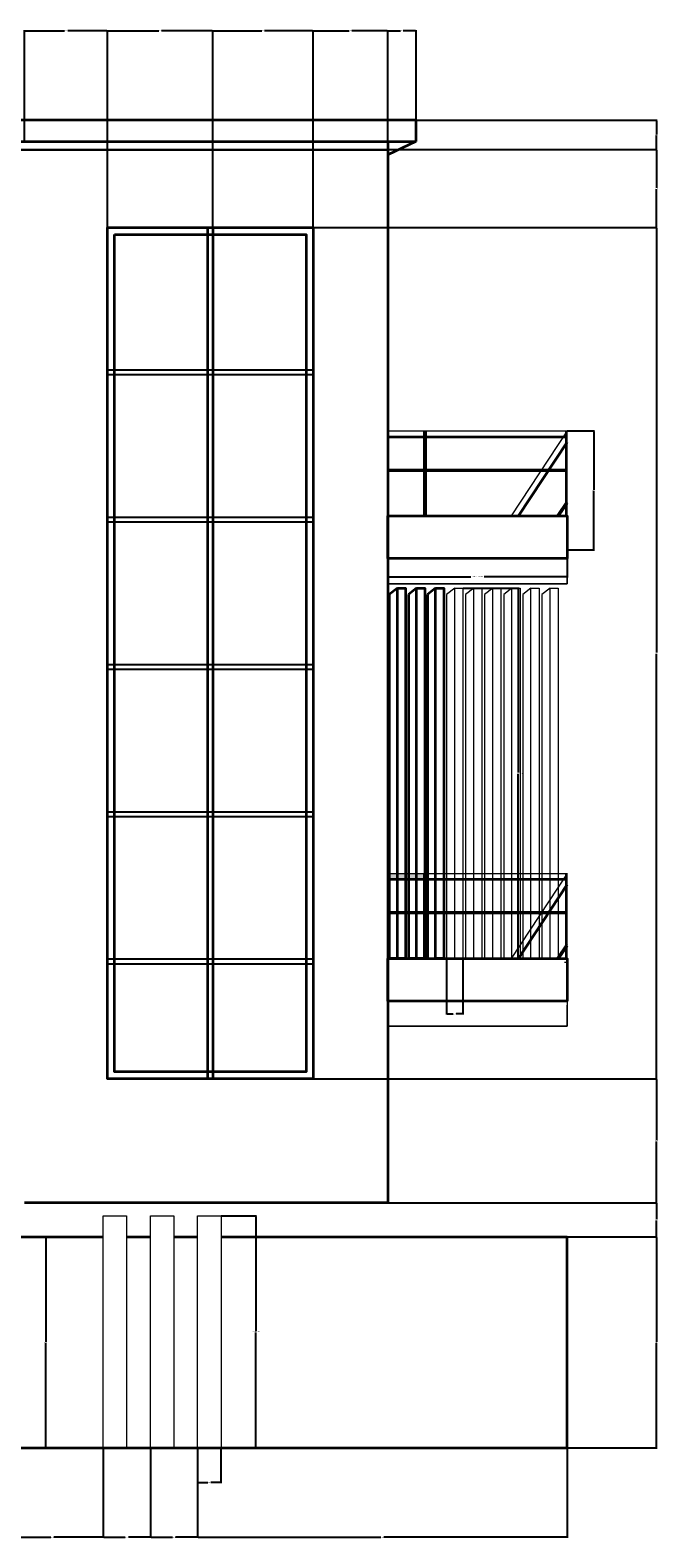
# Model space of a CAD drawing. Units: feet. Extents: x 2415 to 6174, y 866 to 1295.
# Tile 8 of 9: x 4309 to 4488, y 866 to 1295. Entities that reach past the tile are written whole.
import ezdxf

# ---------------------------------------------------------------- set-up
doc = ezdxf.new("R2010")
doc.units = ezdxf.units.FT
for name, color, linetype, lineweight in [('A-ANNO-DIMS', 2, 'Continuous', 18), ('A-ELEV', 7, 'Continuous', 35), ('A-ELEV-LOUV', 9, 'Continuous', 18), ('A-ELEV-PATT', 8, 'Continuous', 13), ('A-ELEV-RAIL', 3, 'Continuous', 18), ('A-GLAZ', 4, 'Continuous', 25)]:
    doc.layers.add(name, color=color, linetype=linetype, lineweight=lineweight)
doc.styles.get("Standard").update_dxf_attribs({"font": 'arial.ttf'})
doc.dimstyles.get("Standard").update_dxf_attribs({"dimtxt": 0.18, "dimasz": 0.18, "dimexe": 0.18, "dimexo": 0.0625, "dimgap": 0.09, "dimtad": 0, "dimtih": 1, "dimtoh": 1, "dimdec": 1, "dimzin": 0, "dimdsep": 46, "dimlunit": 3, "dimtxsty": 'Standard', "dimcen": 0.09, "dimadec": 0, "dimazin": 0, "dimtfac": 1, "dimtdec": 1, "dimtofl": 0, "dimtmove": 0, "dimatfit": 3, "dimfxl": 1, "dimtolj": 1, "dimtzin": 0, "dimarcsym": 0})

# ---------------------------------------------------------------- blocks, each defined once
blk = doc.blocks.new('LOUVER-SLAT')
for p, q in [((2.33, 105.44), (0, 103.66)), ((0, 103.66), (0, 0))]:
    blk.add_line(p, q)
blk.add_lwpolyline([(2.33, 105.44), (4.65, 105.44), (4.65, 0), (2.33, 0)], close=True)
blk = doc.blocks.new('FACADE-FIN')
blk.add_line((0, 66), (6.66, 66))
for points in [[(0, 0), (0, 66)], [(6.66, 66), (6.66, 0)]]:
    blk.add_lwpolyline(points)
blk = doc.blocks.new('BALCONY-RAIL-PANEL')
for p, q in [((51.06, 33.86), (35.09, 9.65)), ((51.06, 0), (51.06, 33.86))]:
    blk.add_line(p, q)
for points in [[(0, 33.86), (51.06, 33.86)], [(50.67, 9.65), (50.67, 33.86)], [(51.06, 33.54), (50.91, 33.64)], [(50.93, 33.86), (50.93, 9.65)]]:
    blk.add_lwpolyline(points)
blk = doc.blocks.new('BALCONY-RAIL-BASE')
for p, q in [((51.06, 0), (51.06, 6)), ((0, 0), (51.06, 0))]:
    blk.add_line(p, q)
blk.add_lwpolyline([(51.06, 0), (0, 0), (0, 7.19), (51.06, 7.19)], close=True)
blk = doc.blocks.new('*D7')
at = {"layer": 'A-ANNO-DIMS', "color": 0, "lineweight": -2, "transparency": 16777216}
for p, q in [((4432.55, 1136.37), (4448.48, 1136.37)), ((4448.3, 1136.19), (4448.3, 1083.83)), ((4448.3, 1031.11), (4448.3, 1083.47)), ((4432.55, 1030.93), (4448.48, 1030.93))]:
    blk.add_line(p, q, dxfattribs=at)
at = {"layer": 'A-ANNO-DIMS', "color": 0, "transparency": 16777216}
for points in [[(4448.27, 1136.19), (4448.33, 1136.19), (4448.3, 1136.37)], [(4448.27, 1031.11), (4448.33, 1031.11), (4448.3, 1030.93)]]:
    blk.add_solid(points, dxfattribs=at)
at = {"layer": 'Defpoints', "color": 0, "transparency": 16777216}
for p in [(4432.49, 1136.37), (4448.3, 1136.37), (4432.49, 1030.93)]:
    blk.add_point(p, dxfattribs=at)
at = {"layer": 'A-ANNO-DIMS', "color": 0, "transparency": 16777216, "insert": (4448.3, 1083.65), "char_height": 0.18, "attachment_point": 5}
blk.add_mtext('\\A1;LOUVER SLAT 105 TYP.', dxfattribs=at)
blk = doc.blocks.new('*D8')
at = {"layer": 'A-ANNO-DIMS', "color": 0, "lineweight": -2, "transparency": 16777216}
for p, q in [((4427.84, 1030.87), (4427.84, 1014.94)), ((4432.49, 1030.87), (4432.49, 1014.94)), ((4428.02, 1015.12), (4429.7, 1015.12)), ((4432.31, 1015.12), (4430.62, 1015.12))]:
    blk.add_line(p, q, dxfattribs=at)
at = {"layer": 'A-ANNO-DIMS', "color": 0, "transparency": 16777216}
for points in [[(4428.02, 1015.15), (4428.02, 1015.09), (4427.84, 1015.12)], [(4432.31, 1015.15), (4432.31, 1015.09), (4432.49, 1015.12)]]:
    blk.add_solid(points, dxfattribs=at)
at = {"layer": 'Defpoints', "color": 0, "transparency": 16777216}
for p in [(4427.84, 1030.93), (4432.49, 1030.93), (4432.49, 1015.12)]:
    blk.add_point(p, dxfattribs=at)
at = {"layer": 'A-ANNO-DIMS', "color": 0, "transparency": 16777216, "insert": (4430.16, 1015.12), "char_height": 0.18, "attachment_point": 5}
blk.add_mtext('\\A1;5 TYP.', dxfattribs=at)
blk = doc.blocks.new('*D9')
at = {"layer": 'A-ANNO-DIMS', "color": 0, "lineweight": -2, "transparency": 16777216}
for p, q in [((4363.66, 957.6), (4373.67, 957.6)), ((4373.49, 957.42), (4373.49, 924.78)), ((4373.49, 891.78), (4373.49, 924.42)), ((4363.66, 891.6), (4373.67, 891.6))]:
    blk.add_line(p, q, dxfattribs=at)
at = {"layer": 'A-ANNO-DIMS', "color": 0, "transparency": 16777216}
for points in [[(4373.46, 957.42), (4373.52, 957.42), (4373.49, 957.6)], [(4373.46, 891.78), (4373.52, 891.78), (4373.49, 891.6)]]:
    blk.add_solid(points, dxfattribs=at)
at = {"layer": 'Defpoints', "color": 0, "transparency": 16777216}
for p in [(4363.59, 957.6), (4373.49, 957.6), (4363.59, 891.6)]:
    blk.add_point(p, dxfattribs=at)
at = {"layer": 'A-ANNO-DIMS', "color": 0, "transparency": 16777216, "insert": (4373.49, 924.6), "char_height": 0.18, "attachment_point": 5}
blk.add_mtext('\\A1;FACADE FIN 66 TYP.', dxfattribs=at)
blk = doc.blocks.new('*D10')
at = {"layer": 'A-ANNO-DIMS', "color": 0, "lineweight": -2, "transparency": 16777216}
for p, q in [((4356.94, 891.54), (4356.94, 881.52)), ((4363.59, 891.54), (4363.59, 881.52)), ((4357.12, 881.7), (4359.81, 881.7)), ((4363.41, 881.7), (4360.72, 881.7))]:
    blk.add_line(p, q, dxfattribs=at)
at = {"layer": 'A-ANNO-DIMS', "color": 0, "transparency": 16777216}
for points in [[(4357.12, 881.73), (4357.12, 881.67), (4356.94, 881.7)], [(4363.41, 881.73), (4363.41, 881.67), (4363.59, 881.7)]]:
    blk.add_solid(points, dxfattribs=at)
at = {"layer": 'Defpoints', "color": 0, "transparency": 16777216}
for p in [(4356.94, 891.6), (4363.59, 891.6), (4363.59, 881.7)]:
    blk.add_point(p, dxfattribs=at)
at = {"layer": 'A-ANNO-DIMS', "color": 0, "transparency": 16777216, "insert": (4360.26, 881.7), "char_height": 0.18, "attachment_point": 5}
blk.add_mtext('\\A1;7 TYP.', dxfattribs=at)
blk = doc.blocks.new('*D11')
at = {"layer": 'A-ANNO-DIMS', "color": 0, "lineweight": -2, "transparency": 16777216}
for p, q in [((4411.13, 1147.22), (4411.13, 1139.44)), ((4462.18, 1147.22), (4462.18, 1139.44)), ((4411.31, 1139.62), (4434.73, 1139.62)), ((4462, 1139.62), (4438.58, 1139.62))]:
    blk.add_line(p, q, dxfattribs=at)
at = {"layer": 'A-ANNO-DIMS', "color": 0, "transparency": 16777216}
for points in [[(4411.31, 1139.65), (4411.31, 1139.59), (4411.13, 1139.62)], [(4462, 1139.65), (4462, 1139.59), (4462.18, 1139.62)]]:
    blk.add_solid(points, dxfattribs=at)
at = {"layer": 'Defpoints', "color": 0, "transparency": 16777216}
for p in [(4411.13, 1147.28), (4462.18, 1147.28), (4462.18, 1139.62)]:
    blk.add_point(p, dxfattribs=at)
at = {"layer": 'A-ANNO-DIMS', "color": 0, "transparency": 16777216, "insert": (4436.66, 1139.62), "char_height": 0.18, "attachment_point": 5}
blk.add_mtext('\\A1;BALCONY RAIL PANEL 51 TYP.', dxfattribs=at)
blk = doc.blocks.new('*D12')
at = {"layer": 'A-ANNO-DIMS', "color": 0, "lineweight": -2, "transparency": 16777216}
for p, q in [((4462.25, 1181.14), (4470.02, 1181.14)), ((4469.84, 1180.96), (4469.84, 1164.39)), ((4469.84, 1147.46), (4469.84, 1164.03)), ((4462.25, 1147.28), (4470.02, 1147.28))]:
    blk.add_line(p, q, dxfattribs=at)
at = {"layer": 'A-ANNO-DIMS', "color": 0, "transparency": 16777216}
for points in [[(4469.81, 1180.96), (4469.87, 1180.96), (4469.84, 1181.14)], [(4469.81, 1147.46), (4469.87, 1147.46), (4469.84, 1147.28)]]:
    blk.add_solid(points, dxfattribs=at)
at = {"layer": 'Defpoints', "color": 0, "transparency": 16777216}
for p in [(4462.18, 1181.14), (4469.84, 1181.14), (4462.18, 1147.28)]:
    blk.add_point(p, dxfattribs=at)
at = {"layer": 'A-ANNO-DIMS', "color": 0, "transparency": 16777216, "insert": (4469.84, 1164.21), "char_height": 0.18, "attachment_point": 5}
blk.add_mtext('\\A1;34 TYP.', dxfattribs=at)
blk = doc.blocks.new('*D16')
at = {"layer": 'A-ANNO-DIMS', "color": 0, "lineweight": -2, "transparency": 16777216}
for p, q in [((4295.05, 951.6), (4313.86, 951.6)), ((4313.68, 951.42), (4313.68, 921.78)), ((4313.68, 891.78), (4313.68, 921.42)), ((4295.05, 891.6), (4313.86, 891.6))]:
    blk.add_line(p, q, dxfattribs=at)
at = {"layer": 'A-ANNO-DIMS', "color": 0, "transparency": 16777216}
for points in [[(4313.65, 951.42), (4313.71, 951.42), (4313.68, 951.6)], [(4313.65, 891.78), (4313.71, 891.78), (4313.68, 891.6)]]:
    blk.add_solid(points, dxfattribs=at)
at = {"layer": 'Defpoints', "color": 0, "transparency": 16777216}
for p in [(4294.99, 951.6), (4313.68, 951.6), (4294.99, 891.6)]:
    blk.add_point(p, dxfattribs=at)
at = {"layer": 'A-ANNO-DIMS', "color": 0, "transparency": 16777216, "insert": (4313.68, 921.6), "char_height": 0.18, "attachment_point": 5}
blk.add_mtext('\\A1;60 TYP.', dxfattribs=at)
blk = doc.blocks.new('*D23')
at = {"layer": 'A-ANNO-DIMS', "color": 0, "lineweight": -2, "transparency": 16777216}
for p, q in [((4300.99, 891.54), (4300.99, 865.92)), ((4330.05, 891.54), (4330.05, 865.92)), ((4301.17, 866.1), (4315.13, 866.1)), ((4329.87, 866.1), (4315.92, 866.1))]:
    blk.add_line(p, q, dxfattribs=at)
at = {"layer": 'A-ANNO-DIMS', "color": 0, "transparency": 16777216}
for points in [[(4301.17, 866.13), (4301.17, 866.07), (4300.99, 866.1)], [(4329.87, 866.13), (4329.87, 866.07), (4330.05, 866.1)]]:
    blk.add_solid(points, dxfattribs=at)
at = {"layer": 'Defpoints', "color": 0, "transparency": 16777216}
for p in [(4300.99, 891.6), (4330.05, 891.6), (4330.05, 866.1)]:
    blk.add_point(p, dxfattribs=at)
at = {"layer": 'A-ANNO-DIMS', "color": 0, "transparency": 16777216, "insert": (4315.52, 866.1), "char_height": 0.18, "attachment_point": 5}
blk.add_mtext('\\A1;29.06', dxfattribs=at)
blk = doc.blocks.new('*D24')
at = {"layer": 'A-ANNO-DIMS', "color": 0, "lineweight": -2, "transparency": 16777216}
for p, q in [((4330.05, 891.54), (4330.05, 865.92)), ((4343.49, 891.54), (4343.49, 865.92)), ((4330.23, 866.1), (4336.32, 866.1)), ((4343.31, 866.1), (4337.23, 866.1))]:
    blk.add_line(p, q, dxfattribs=at)
at = {"layer": 'A-ANNO-DIMS', "color": 0, "transparency": 16777216}
for points in [[(4330.23, 866.13), (4330.23, 866.07), (4330.05, 866.1)], [(4343.31, 866.13), (4343.31, 866.07), (4343.49, 866.1)]]:
    blk.add_solid(points, dxfattribs=at)
at = {"layer": 'Defpoints', "color": 0, "transparency": 16777216}
for p in [(4330.05, 891.6), (4343.49, 891.6), (4343.49, 866.1)]:
    blk.add_point(p, dxfattribs=at)
at = {"layer": 'A-ANNO-DIMS', "color": 0, "transparency": 16777216, "insert": (4336.77, 866.1), "char_height": 0.18, "attachment_point": 5}
blk.add_mtext('\\A1;13.442', dxfattribs=at)
blk = doc.blocks.new('*D25')
at = {"layer": 'A-ANNO-DIMS', "color": 0, "lineweight": -2, "transparency": 16777216}
for p, q in [((4343.49, 891.54), (4343.49, 865.92)), ((4356.94, 891.54), (4356.94, 865.92)), ((4343.67, 866.1), (4349.76, 866.1)), ((4356.76, 866.1), (4350.67, 866.1))]:
    blk.add_line(p, q, dxfattribs=at)
at = {"layer": 'A-ANNO-DIMS', "color": 0, "transparency": 16777216}
for points in [[(4343.67, 866.13), (4343.67, 866.07), (4343.49, 866.1)], [(4356.76, 866.13), (4356.76, 866.07), (4356.94, 866.1)]]:
    blk.add_solid(points, dxfattribs=at)
at = {"layer": 'Defpoints', "color": 0, "transparency": 16777216}
for p in [(4343.49, 891.6), (4356.94, 891.6), (4356.94, 866.1)]:
    blk.add_point(p, dxfattribs=at)
at = {"layer": 'A-ANNO-DIMS', "color": 0, "transparency": 16777216, "insert": (4350.21, 866.1), "char_height": 0.18, "attachment_point": 5}
blk.add_mtext('\\A1;13.442', dxfattribs=at)
blk = doc.blocks.new('*D26')
at = {"layer": 'A-ANNO-DIMS', "color": 0, "lineweight": -2, "transparency": 16777216}
for p, q in [((4356.94, 891.54), (4356.94, 865.92)), ((4462.18, 891.54), (4462.18, 865.92)), ((4357.12, 866.1), (4409.1, 866.1)), ((4462, 866.1), (4410.02, 866.1))]:
    blk.add_line(p, q, dxfattribs=at)
at = {"layer": 'A-ANNO-DIMS', "color": 0, "transparency": 16777216}
for points in [[(4357.12, 866.13), (4357.12, 866.07), (4356.94, 866.1)], [(4462, 866.13), (4462, 866.07), (4462.18, 866.1)]]:
    blk.add_solid(points, dxfattribs=at)
at = {"layer": 'Defpoints', "color": 0, "transparency": 16777216}
for p in [(4356.94, 891.6), (4462.18, 891.6), (4462.18, 866.1)]:
    blk.add_point(p, dxfattribs=at)
at = {"layer": 'A-ANNO-DIMS', "color": 0, "transparency": 16777216, "insert": (4409.56, 866.1), "char_height": 0.18, "attachment_point": 5}
blk.add_mtext('\\A1;105.25', dxfattribs=at)
blk = doc.blocks.new('*D33')
at = {"layer": 'A-ANNO-DIMS', "color": 0, "lineweight": -2, "transparency": 16777216}
for p, q in [((4307.61, 1263.66), (4307.61, 1295.28)), ((4307.79, 1295.1), (4318.98, 1295.1)), ((4331.09, 1295.1), (4319.91, 1295.1)), ((4331.27, 1239.13), (4331.27, 1295.28))]:
    blk.add_line(p, q, dxfattribs=at)
at = {"layer": 'A-ANNO-DIMS', "color": 0, "transparency": 16777216}
for points in [[(4307.79, 1295.13), (4307.79, 1295.07), (4307.61, 1295.1)], [(4331.09, 1295.13), (4331.09, 1295.07), (4331.27, 1295.1)]]:
    blk.add_solid(points, dxfattribs=at)
at = {"layer": 'Defpoints', "color": 0, "transparency": 16777216}
for p in [(4331.27, 1295.1), (4307.61, 1263.6), (4331.27, 1239.07)]:
    blk.add_point(p, dxfattribs=at)
at = {"layer": 'A-ANNO-DIMS', "color": 0, "transparency": 16777216, "insert": (4319.44, 1295.1), "char_height": 0.18, "attachment_point": 5}
blk.add_mtext('\\A1;23.657', dxfattribs=at)
blk = doc.blocks.new('*D34')
at = {"layer": 'A-ANNO-DIMS', "color": 0, "lineweight": -2, "transparency": 16777216}
for p, q in [((4331.27, 1239.13), (4331.27, 1295.28)), ((4331.45, 1295.1), (4345.89, 1295.1)), ((4361.12, 1295.1), (4346.68, 1295.1)), ((4361.3, 1239.13), (4361.3, 1295.28))]:
    blk.add_line(p, q, dxfattribs=at)
at = {"layer": 'A-ANNO-DIMS', "color": 0, "transparency": 16777216}
for points in [[(4331.45, 1295.13), (4331.45, 1295.07), (4331.27, 1295.1)], [(4361.12, 1295.13), (4361.12, 1295.07), (4361.3, 1295.1)]]:
    blk.add_solid(points, dxfattribs=at)
at = {"layer": 'Defpoints', "color": 0, "transparency": 16777216}
for p in [(4361.3, 1295.1), (4331.27, 1239.07), (4361.3, 1239.07)]:
    blk.add_point(p, dxfattribs=at)
at = {"layer": 'A-ANNO-DIMS', "color": 0, "transparency": 16777216, "insert": (4346.29, 1295.1), "char_height": 0.18, "attachment_point": 5}
blk.add_mtext('\\A1;30.03', dxfattribs=at)
blk = doc.blocks.new('*D35')
at = {"layer": 'A-ANNO-DIMS', "color": 0, "lineweight": -2, "transparency": 16777216}
for p, q in [((4361.3, 1239.13), (4361.3, 1295.28)), ((4361.48, 1295.1), (4375.19, 1295.1)), ((4389.69, 1295.1), (4375.98, 1295.1)), ((4389.87, 1239.13), (4389.87, 1295.28))]:
    blk.add_line(p, q, dxfattribs=at)
at = {"layer": 'A-ANNO-DIMS', "color": 0, "transparency": 16777216}
for points in [[(4361.48, 1295.13), (4361.48, 1295.07), (4361.3, 1295.1)], [(4389.69, 1295.13), (4389.69, 1295.07), (4389.87, 1295.1)]]:
    blk.add_solid(points, dxfattribs=at)
at = {"layer": 'Defpoints', "color": 0, "transparency": 16777216}
for p in [(4389.87, 1295.1), (4361.3, 1239.07), (4389.87, 1239.07)]:
    blk.add_point(p, dxfattribs=at)
at = {"layer": 'A-ANNO-DIMS', "color": 0, "transparency": 16777216, "insert": (4375.58, 1295.1), "char_height": 0.18, "attachment_point": 5}
blk.add_mtext('\\A1;28.57', dxfattribs=at)
blk = doc.blocks.new('*D36')
at = {"layer": 'A-ANNO-DIMS', "color": 0, "lineweight": -2, "transparency": 16777216}
for p, q in [((4389.87, 1239.13), (4389.87, 1295.28)), ((4390.05, 1295.1), (4400.1, 1295.1)), ((4410.95, 1295.1), (4400.89, 1295.1)), ((4411.13, 1261.33), (4411.13, 1295.28))]:
    blk.add_line(p, q, dxfattribs=at)
at = {"layer": 'A-ANNO-DIMS', "color": 0, "transparency": 16777216}
for points in [[(4390.05, 1295.13), (4390.05, 1295.07), (4389.87, 1295.1)], [(4410.95, 1295.13), (4410.95, 1295.07), (4411.13, 1295.1)]]:
    blk.add_solid(points, dxfattribs=at)
at = {"layer": 'Defpoints', "color": 0, "transparency": 16777216}
for p in [(4411.13, 1295.1), (4411.13, 1261.26), (4389.87, 1239.07)]:
    blk.add_point(p, dxfattribs=at)
at = {"layer": 'A-ANNO-DIMS', "color": 0, "transparency": 16777216, "insert": (4400.5, 1295.1), "char_height": 0.18, "attachment_point": 5}
blk.add_mtext('\\A1;21.26', dxfattribs=at)
blk = doc.blocks.new('*D37')
at = {"layer": 'A-ANNO-DIMS', "color": 0, "lineweight": -2, "transparency": 16777216}
for p, q in [((4411.13, 1261.33), (4411.13, 1295.28)), ((4411.31, 1295.1), (4414.74, 1295.1)), ((4418.97, 1295.1), (4415.53, 1295.1)), ((4419.15, 1269.66), (4419.15, 1295.28))]:
    blk.add_line(p, q, dxfattribs=at)
at = {"layer": 'A-ANNO-DIMS', "color": 0, "transparency": 16777216}
for points in [[(4411.31, 1295.13), (4411.31, 1295.07), (4411.13, 1295.1)], [(4418.97, 1295.13), (4418.97, 1295.07), (4419.15, 1295.1)]]:
    blk.add_solid(points, dxfattribs=at)
at = {"layer": 'Defpoints', "color": 0, "transparency": 16777216}
for p in [(4419.15, 1295.1), (4419.15, 1269.6), (4411.13, 1261.26)]:
    blk.add_point(p, dxfattribs=at)
at = {"layer": 'A-ANNO-DIMS', "color": 0, "transparency": 16777216, "insert": (4415.14, 1295.1), "char_height": 0.18, "attachment_point": 5}
blk.add_mtext('\\A1;8.019', dxfattribs=at)
blk = doc.blocks.new('*D45')
at = {"layer": 'A-ANNO-DIMS', "color": 0, "lineweight": -2, "transparency": 16777216}
for p, q in [((4462.25, 951.6), (4487.86, 951.6)), ((4487.68, 951.42), (4487.68, 921.78)), ((4487.68, 891.78), (4487.68, 921.42)), ((4462.25, 891.6), (4487.86, 891.6))]:
    blk.add_line(p, q, dxfattribs=at)
at = {"layer": 'A-ANNO-DIMS', "color": 0, "transparency": 16777216}
for points in [[(4487.65, 951.42), (4487.71, 951.42), (4487.68, 951.6)], [(4487.65, 891.78), (4487.71, 891.78), (4487.68, 891.6)]]:
    blk.add_solid(points, dxfattribs=at)
at = {"layer": 'Defpoints', "color": 0, "transparency": 16777216}
for p in [(4462.18, 951.6), (4487.68, 951.6), (4462.18, 891.6)]:
    blk.add_point(p, dxfattribs=at)
at = {"layer": 'A-ANNO-DIMS', "color": 0, "transparency": 16777216, "insert": (4487.68, 921.6), "char_height": 0.18, "attachment_point": 5}
blk.add_mtext('\\A1;60', dxfattribs=at)
blk = doc.blocks.new('*D46')
at = {"layer": 'A-ANNO-DIMS', "color": 0, "lineweight": -2, "transparency": 16777216}
for p, q in [((4411.19, 961.37), (4487.86, 961.37)), ((4487.68, 961.19), (4487.68, 956.66)), ((4487.68, 951.78), (4487.68, 956.3)), ((4462.25, 951.6), (4487.86, 951.6))]:
    blk.add_line(p, q, dxfattribs=at)
at = {"layer": 'A-ANNO-DIMS', "color": 0, "transparency": 16777216}
for points in [[(4487.65, 961.19), (4487.71, 961.19), (4487.68, 961.37)], [(4487.65, 951.78), (4487.71, 951.78), (4487.68, 951.6)]]:
    blk.add_solid(points, dxfattribs=at)
at = {"layer": 'Defpoints', "color": 0, "transparency": 16777216}
for p in [(4411.13, 961.37), (4487.68, 961.37), (4462.18, 951.6)]:
    blk.add_point(p, dxfattribs=at)
at = {"layer": 'A-ANNO-DIMS', "color": 0, "transparency": 16777216, "insert": (4487.68, 956.48), "char_height": 0.18, "attachment_point": 5}
blk.add_mtext('\\A1;9.766', dxfattribs=at)
blk = doc.blocks.new('*D47')
at = {"layer": 'A-ANNO-DIMS', "color": 0, "lineweight": -2, "transparency": 16777216}
for p, q in [((4389.93, 996.64), (4487.86, 996.64)), ((4487.68, 996.46), (4487.68, 979.19)), ((4487.68, 961.55), (4487.68, 978.82)), ((4411.19, 961.37), (4487.86, 961.37))]:
    blk.add_line(p, q, dxfattribs=at)
at = {"layer": 'A-ANNO-DIMS', "color": 0, "transparency": 16777216}
for points in [[(4487.65, 996.46), (4487.71, 996.46), (4487.68, 996.64)], [(4487.65, 961.55), (4487.71, 961.55), (4487.68, 961.37)]]:
    blk.add_solid(points, dxfattribs=at)
at = {"layer": 'Defpoints', "color": 0, "transparency": 16777216}
for p in [(4389.87, 996.64), (4487.68, 996.64), (4411.13, 961.37)]:
    blk.add_point(p, dxfattribs=at)
at = {"layer": 'A-ANNO-DIMS', "color": 0, "transparency": 16777216, "insert": (4487.68, 979.01), "char_height": 0.18, "attachment_point": 5}
blk.add_mtext('\\A1;35.28', dxfattribs=at)
blk = doc.blocks.new('*D48')
at = {"layer": 'A-ANNO-DIMS', "color": 0, "lineweight": -2, "transparency": 16777216}
for p, q in [((4389.93, 1239.07), (4487.86, 1239.07)), ((4487.68, 1238.89), (4487.68, 1118.04)), ((4487.68, 996.82), (4487.68, 1117.68)), ((4389.93, 996.64), (4487.86, 996.64))]:
    blk.add_line(p, q, dxfattribs=at)
at = {"layer": 'A-ANNO-DIMS', "color": 0, "transparency": 16777216}
for points in [[(4487.65, 1238.89), (4487.71, 1238.89), (4487.68, 1239.07)], [(4487.65, 996.82), (4487.71, 996.82), (4487.68, 996.64)]]:
    blk.add_solid(points, dxfattribs=at)
at = {"layer": 'Defpoints', "color": 0, "transparency": 16777216}
for p in [(4389.87, 1239.07), (4487.68, 1239.07), (4389.87, 996.64)]:
    blk.add_point(p, dxfattribs=at)
at = {"layer": 'A-ANNO-DIMS', "color": 0, "transparency": 16777216, "insert": (4487.68, 1117.86), "char_height": 0.18, "attachment_point": 5}
blk.add_mtext('\\A1;242.4', dxfattribs=at)
blk = doc.blocks.new('*D49')
at = {"layer": 'A-ANNO-DIMS', "color": 0, "lineweight": -2, "transparency": 16777216}
for p, q in [((4411.19, 1261.26), (4487.86, 1261.26)), ((4487.68, 1261.08), (4487.68, 1250.35)), ((4487.68, 1239.25), (4487.68, 1249.98)), ((4389.93, 1239.07), (4487.86, 1239.07))]:
    blk.add_line(p, q, dxfattribs=at)
at = {"layer": 'A-ANNO-DIMS', "color": 0, "transparency": 16777216}
for points in [[(4487.65, 1261.08), (4487.71, 1261.08), (4487.68, 1261.26)], [(4487.65, 1239.25), (4487.71, 1239.25), (4487.68, 1239.07)]]:
    blk.add_solid(points, dxfattribs=at)
at = {"layer": 'Defpoints', "color": 0, "transparency": 16777216}
for p in [(4411.13, 1261.26), (4487.68, 1261.26), (4389.87, 1239.07)]:
    blk.add_point(p, dxfattribs=at)
at = {"layer": 'A-ANNO-DIMS', "color": 0, "transparency": 16777216, "insert": (4487.68, 1250.16), "char_height": 0.18, "attachment_point": 5}
blk.add_mtext('\\A1;22.196', dxfattribs=at)
blk = doc.blocks.new('*D50')
at = {"layer": 'A-ANNO-DIMS', "color": 0, "lineweight": -2, "transparency": 16777216}
for p, q in [((4419.21, 1269.6), (4487.86, 1269.6)), ((4487.68, 1269.42), (4487.68, 1265.61)), ((4487.68, 1261.44), (4487.68, 1265.25)), ((4411.19, 1261.26), (4487.86, 1261.26))]:
    blk.add_line(p, q, dxfattribs=at)
at = {"layer": 'A-ANNO-DIMS', "color": 0, "transparency": 16777216}
for points in [[(4487.65, 1269.42), (4487.71, 1269.42), (4487.68, 1269.6)], [(4487.65, 1261.44), (4487.71, 1261.44), (4487.68, 1261.26)]]:
    blk.add_solid(points, dxfattribs=at)
at = {"layer": 'Defpoints', "color": 0, "transparency": 16777216}
for p in [(4419.15, 1269.6), (4487.68, 1269.6), (4411.13, 1261.26)]:
    blk.add_point(p, dxfattribs=at)
at = {"layer": 'A-ANNO-DIMS', "color": 0, "transparency": 16777216, "insert": (4487.68, 1265.43), "char_height": 0.18, "attachment_point": 5}
blk.add_mtext('\\A1;8.336', dxfattribs=at)

msp = doc.modelspace()

# ---------------------------------------------------------------- hatches: boundary and pattern name
at = {"layer": 'A-ELEV-PATT'}
h = msp.add_hatch(color=256, dxfattribs=at)
h.set_gradient(color2=(0, 0, 0))
h.paths.add_polyline_path([(4413.8595, 1055.1411), (4411.5333, 1055.1411), (4411.5333, 1053.3943), (4413.8595, 1053.3943)])
h.paths.add_polyline_path([(4411.5333, 1055.1411), (4411.1278, 1055.1411), (4411.1278, 1053.3943), (4411.5333, 1053.3943)])
h.paths.add_polyline_path([(4416.1857, 1055.1411), (4413.8595, 1055.1411), (4413.8595, 1053.3943), (4416.1857, 1053.3943)])
h.paths.add_polyline_path([(4416.9678, 1055.1411), (4416.1857, 1055.1411), (4416.1857, 1053.3943), (4416.9678, 1053.3943)])
h.paths.add_polyline_path([(4419.294, 1055.1411), (4416.9678, 1055.1411), (4416.9678, 1053.3943), (4419.294, 1053.3943)])
h.paths.add_polyline_path([(4421.5982, 1055.1411), (4419.294, 1055.1411), (4419.294, 1053.3943), (4421.5982, 1053.3943)])

# ---------------------------------------------------------------- linework, layer by layer
at = {"layer": 'A-ELEV'}
for p, q in [((4419.1468, 1269.5992), (4300.9903, 1269.5992)), ((4419.1468, 1269.5992), (4419.1468, 1263.5992)), ((4300.9903, 1263.5992), (4419.1468, 1263.5992)), ((4419.1468, 1263.5992), (4411.1278, 1259.8122)), ((4300.9903, 1261.2303), (4411.1278, 1261.2628)), ((4413.8595, 1136.3701), (4411.5333, 1134.5952)), ((4411.5333, 1134.5952), (4411.5333, 1030.9315)), ((4419.294, 1136.3701), (4416.9678, 1134.5952)), ((4416.9678, 1134.5952), (4416.9678, 1030.9315)), ((4424.7285, 1136.3701), (4422.4023, 1134.5952)), ((4422.4023, 1134.5952), (4422.4023, 1030.9315)), ((4413.8595, 1030.9315), (4411.5333, 1030.9315)), ((4419.294, 1030.9315), (4416.9678, 1030.9315)), ((4300.9903, 951.5992), (4330.0513, 951.5992)), ((4336.7088, 951.5992), (4343.4934, 951.5992)), ((4350.1509, 951.5992), (4356.9355, 951.5992)), ((4363.593, 951.5992), (4462.1845, 951.5992)), ((4462.1845, 891.5992), (4462.1845, 951.5992)), ((3982.1845, 891.5992), (4462.1845, 891.5992))]:
    msp.add_line(p, q, dxfattribs=at)
for points in [[(4411.1278, 1263.5992), (4411.1278, 961.3655), (4307.6134, 961.3655)], [(4421.5982, 1156.9315), (4421.5982, 1181.1411)], [(4421.8621, 1181.1411), (4421.8621, 1156.9315)], [(4462.1845, 1179.3943), (4411.1278, 1179.3943)], [(4462.1845, 1177.9687), (4448.3083, 1156.9315)], [(4411.1278, 1170.0699), (4462.1845, 1170.0699)], [(4462.1845, 1169.806), (4411.1278, 1169.806)], [(4459.4784, 1156.9315), (4462.1845, 1161.0342)], [(4462.1845, 1160.5548), (4459.7946, 1156.9315)], [(4462.1845, 1053.3943), (4411.1278, 1053.3943)], [(4421.5982, 1030.9315), (4421.5982, 1055.1411)], [(4421.8621, 1055.1411), (4421.8621, 1030.9315)], [(4462.1845, 1051.9687), (4448.3083, 1030.9315)], [(4411.1278, 1044.0699), (4462.1845, 1044.0699)], [(4462.1845, 1043.806), (4411.1278, 1043.806)], [(4459.4784, 1030.9315), (4462.1845, 1035.0342)], [(4462.1845, 1034.5548), (4459.7946, 1030.9315)], [(4461.798, 1029.6456), (4461.798, 1029.9095)], [(4462.062, 1029.9095), (4462.062, 1029.6456)]]:
    msp.add_lwpolyline(points, dxfattribs=at)
for points in [[(4331.2706, 1239.0671), (4389.8684, 1239.0671), (4389.8684, 996.6447), (4331.2706, 996.6447)], [(4333.2706, 1237.0671), (4387.8684, 1237.0671), (4387.8684, 998.6447), (4333.2706, 998.6447)], [(4359.8388, 1239.0671), (4361.3002, 1239.0671), (4361.3002, 996.6447), (4359.8388, 996.6447)], [(4462.1845, 1144.7857), (4411.1278, 1144.7857), (4411.1278, 1156.9315), (4462.1845, 1156.9315)], [(4413.8595, 1136.3701), (4416.1857, 1136.3701), (4416.1857, 1030.9315), (4413.8595, 1030.9315)], [(4419.294, 1136.3701), (4421.6202, 1136.3701), (4421.6202, 1030.9315), (4419.294, 1030.9315)], [(4424.7285, 1136.3701), (4427.0547, 1136.3701), (4427.0547, 1030.9315), (4424.7285, 1030.9315)], [(4462.1845, 1018.7857), (4411.1278, 1018.7857), (4411.1278, 1030.9315), (4462.1845, 1030.9315)]]:
    msp.add_lwpolyline(points, close=True, dxfattribs=at)
at = {"layer": 'A-GLAZ'}
for points in [[(4389.8684, 1197.114), (4331.2706, 1197.114), (4331.2706, 1198.5754), (4389.8684, 1198.5754)], [(4389.8684, 1155.161), (4331.2706, 1155.161), (4331.2706, 1156.6224), (4389.8684, 1156.6224)], [(4389.8684, 1113.2079), (4331.2706, 1113.2079), (4331.2706, 1114.6693), (4389.8684, 1114.6693)], [(4389.8684, 1071.2549), (4331.2706, 1071.2549), (4331.2706, 1072.7163), (4389.8684, 1072.7163)], [(4389.8684, 1029.3019), (4331.2706, 1029.3019), (4331.2706, 1030.7632), (4389.8684, 1030.7632)]]:
    msp.add_lwpolyline(points, dxfattribs=at)

# ---------------------------------------------------------------- block references
at = {"layer": 'A-ELEV-LOUV'}
for name, p in [('LOUVER-SLAT', (4427.8371, 1030.932)), ('LOUVER-SLAT', (4433.2716, 1030.932)), ('LOUVER-SLAT', (4438.706, 1030.932)), ('LOUVER-SLAT', (4444.1405, 1030.932)), ('LOUVER-SLAT', (4449.575, 1030.932)), ('LOUVER-SLAT', (4455.0095, 1030.932)), ('FACADE-FIN', (4330.0514, 891.599)), ('FACADE-FIN', (4343.4935, 891.599)), ('FACADE-FIN', (4356.9356, 891.599))]:
    msp.add_blockref(name, p, dxfattribs=at)
at = {"layer": 'A-ELEV-RAIL'}
for name, p in [('BALCONY-RAIL-PANEL', (4411.1276, 1147.282)), ('BALCONY-RAIL-BASE', (4411.1276, 1137.599)), ('BALCONY-RAIL-PANEL', (4411.1276, 1021.282)), ('BALCONY-RAIL-BASE', (4411.1276, 1011.599))]:
    msp.add_blockref(name, p, dxfattribs=at)

# ---------------------------------------------------------------- dimensions: what is measured, and where the dimension line sits
at = {"layer": 'A-ANNO-DIMS'}
for base, p1, p2, override, picture, middle in [((4331.2706, 1295.0992), (4307.6134, 1263.5992), (4331.2706, 1239.0671), {"dimdec": 3, "dimlfac": 1, "dimrnd": 0, "dimzin": 0, "dimdsep": 46, "dimlunit": 2}, '*D33', (4319.442, 1295.0992)), ((4361.3002, 1295.0992), (4331.2706, 1239.0671), (4361.3002, 1239.0671), {"dimdec": 2, "dimlfac": 1, "dimrnd": 0, "dimzin": 0, "dimdsep": 46, "dimlunit": 2}, '*D34', (4346.2854, 1295.0992)), ((4389.8684, 1295.0992), (4361.3002, 1239.0671), (4389.8684, 1239.0671), {"dimdec": 2, "dimlfac": 1, "dimrnd": 0, "dimzin": 0, "dimdsep": 46, "dimlunit": 2}, '*D35', (4375.5843, 1295.0992)), ((4411.1278, 1295.0992), (4389.8684, 1239.0671), (4411.1278, 1261.2628), {"dimdec": 2, "dimlfac": 1, "dimrnd": 0, "dimzin": 0, "dimdsep": 46, "dimlunit": 2}, '*D36', (4400.4981, 1295.0992)), ((4419.1468, 1295.0992), (4411.1278, 1261.2628), (4419.1468, 1269.5992), {"dimdec": 3, "dimlfac": 1, "dimrnd": 0, "dimzin": 0, "dimdsep": 46, "dimlunit": 2}, '*D37', (4415.1373, 1295.0992)), ((4330.0513, 866.0992), (4300.9903, 891.5992), (4330.0513, 891.5992), {"dimdec": 2, "dimlfac": 1, "dimrnd": 0, "dimzin": 0, "dimdsep": 46, "dimlunit": 2}, '*D23', (4315.5208, 866.0992)), ((4343.4934, 866.0992), (4330.0513, 891.5992), (4343.4934, 891.5992), {"dimdec": 3, "dimlfac": 1, "dimrnd": 0, "dimzin": 0, "dimdsep": 46, "dimlunit": 2}, '*D24', (4336.7724, 866.0992)), ((4356.9355, 866.0992), (4343.4934, 891.5992), (4356.9355, 891.5992), {"dimdec": 3, "dimlfac": 1, "dimrnd": 0, "dimzin": 0, "dimdsep": 46, "dimlunit": 2}, '*D25', (4350.2145, 866.0992)), ((4462.1845, 866.0992), (4356.9355, 891.5992), (4462.1845, 891.5992), {"dimdec": 2, "dimlfac": 1, "dimrnd": 0, "dimzin": 0, "dimdsep": 46, "dimlunit": 2}, '*D26', (4409.56, 866.0992))]:
    dim = msp.add_linear_dim(base=base, p1=p1, p2=p2, dimstyle='Standard', override=override, dxfattribs=at)
    dim.commit()
    dim.dimension.update_dxf_attribs({"geometry": picture, "text_midpoint": middle})
for base, p1, p2, override, picture, middle in [((4487.6845, 1269.5992), (4411.1278, 1261.2628), (4419.1468, 1269.5992), {"dimdec": 3, "dimlfac": 1, "dimrnd": 0, "dimzin": 0, "dimdsep": 46, "dimlunit": 2}, '*D50', (4487.6845, 1265.431)), ((4487.6845, 1261.2628), (4389.8684, 1239.0671), (4411.1278, 1261.2628), {"dimdec": 3, "dimlfac": 1, "dimrnd": 0, "dimzin": 0, "dimdsep": 46, "dimlunit": 2}, '*D49', (4487.6845, 1250.1649)), ((4487.6845, 1239.0671), (4389.8684, 996.6447), (4389.8684, 1239.0671), {"dimdec": 1, "dimlfac": 1, "dimrnd": 0, "dimzin": 0, "dimdsep": 46, "dimlunit": 2}, '*D48', (4487.6845, 1117.8559)), ((4487.6845, 996.6447), (4411.1278, 961.3655), (4389.8684, 996.6447), {"dimdec": 2, "dimlfac": 1, "dimrnd": 0, "dimzin": 0, "dimdsep": 46, "dimlunit": 2}, '*D47', (4487.6845, 979.0051)), ((4487.6845, 961.3655), (4462.1845, 951.5992), (4411.1278, 961.3655), {"dimdec": 3, "dimlfac": 1, "dimrnd": 0, "dimzin": 0, "dimdsep": 46, "dimlunit": 2}, '*D46', (4487.6845, 956.4824)), ((4487.6845, 951.5992), (4462.1845, 891.5992), (4462.1845, 951.5992), {"dimdec": 0, "dimlfac": 1, "dimrnd": 0, "dimzin": 0, "dimdsep": 46, "dimlunit": 2}, '*D45', (4487.6845, 921.5992))]:
    dim = msp.add_linear_dim(base=base, p1=p1, p2=p2, angle=90, dimstyle='Standard', override=override, dxfattribs=at)
    dim.commit()
    dim.dimension.update_dxf_attribs({"geometry": picture, "text_midpoint": middle})
for base, p1, p2, text, picture, middle in [((4469.8431, 1181.1411), (4462.1845, 1147.2819), (4462.1845, 1181.1411), '<> TYP.', '*D12', (4469.8431, 1164.2115)), ((4448.305, 1136.3701), (4432.4892, 1030.9315), (4432.4892, 1136.3701), 'LOUVER SLAT <> TYP.', '*D7', (4448.305, 1083.6508)), ((4373.493, 957.5993), (4363.593, 891.5992), (4363.593, 957.5993), 'FACADE FIN <> TYP.', '*D9', (4373.493, 924.5993)), ((4313.6843, 951.5992), (4294.9903, 891.5992), (4294.9903, 951.5992), '<> TYP.', '*D16', (4313.6843, 921.5993))]:
    dim = msp.add_linear_dim(base=base, p1=p1, p2=p2, angle=90, text=text, dimstyle='Standard', override={"dimdec": 0, "dimrnd": 0, "dimzin": 0, "dimlunit": 2}, dxfattribs=at)
    dim.commit()
    dim.dimension.update_dxf_attribs({"geometry": picture, "text_midpoint": middle})
for base, p1, p2, text, picture, middle in [((4462.1845, 1139.6233), (4411.1278, 1147.2819), (4462.1845, 1147.2819), 'BALCONY RAIL PANEL <> TYP.', '*D11', (4436.6562, 1139.6233)), ((4432.4892, 1015.1157), (4427.8368, 1030.9315), (4432.4892, 1030.9315), '<> TYP.', '*D8', (4430.163, 1015.1157)), ((4363.593, 881.6993), (4356.9355, 891.5992), (4363.593, 891.5992), '<> TYP.', '*D10', (4360.2642, 881.6993))]:
    dim = msp.add_linear_dim(base=base, p1=p1, p2=p2, text=text, dimstyle='Standard', override={"dimdec": 0, "dimrnd": 0, "dimzin": 0, "dimlunit": 2}, dxfattribs=at)
    dim.commit()
    dim.dimension.update_dxf_attribs({"geometry": picture, "text_midpoint": middle})

doc.saveas('drawing.dxf')
